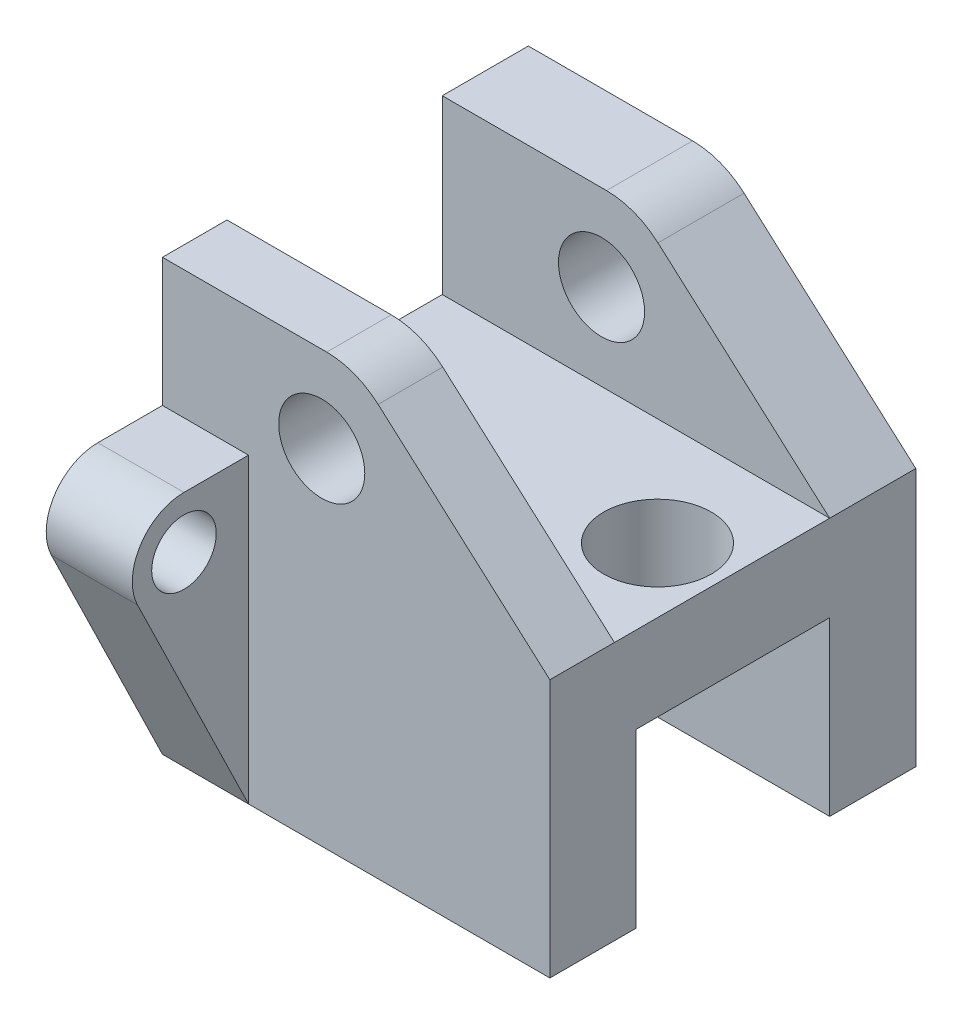
ISO-10303-21;
HEADER;
FILE_DESCRIPTION(('STEP AP214'),'2;1');
FILE_NAME('part.step','',(''),(''),'','','');
FILE_SCHEMA(('AUTOMOTIVE_DESIGN { 1 0 10303 214 1 1 1 1 }'));
ENDSEC;
DATA;
#1=APPLICATION_CONTEXT('core data for automotive mechanical design processes');
#2=APPLICATION_PROTOCOL_DEFINITION('international standard','automotive_design',2000,#1);
#3=PRODUCT_CONTEXT('',#1,'mechanical');
#4=PRODUCT('Part','Part','',(#3));
#5=PRODUCT_RELATED_PRODUCT_CATEGORY('part','',(#4));
#6=PRODUCT_DEFINITION_FORMATION('','',#4);
#7=PRODUCT_DEFINITION_CONTEXT('part definition',#1,'design');
#8=PRODUCT_DEFINITION('design','',#6,#7);
#9=PRODUCT_DEFINITION_SHAPE('','',#8);
#10=(LENGTH_UNIT() NAMED_UNIT(*) SI_UNIT(.MILLI.,.METRE.));
#11=(NAMED_UNIT(*) PLANE_ANGLE_UNIT() SI_UNIT($,.RADIAN.));
#12=(NAMED_UNIT(*) SI_UNIT($,.STERADIAN.) SOLID_ANGLE_UNIT());
#13=UNCERTAINTY_MEASURE_WITH_UNIT(LENGTH_MEASURE(1.E-05),#10,'distance_accuracy_value','');
#14=(GEOMETRIC_REPRESENTATION_CONTEXT(3) GLOBAL_UNCERTAINTY_ASSIGNED_CONTEXT((#13)) GLOBAL_UNIT_ASSIGNED_CONTEXT((#10,
#11,#12)) REPRESENTATION_CONTEXT('',''));
#15=CARTESIAN_POINT('',(0.,0.,0.));
#16=DIRECTION('',(0.,0.,1.));
#17=DIRECTION('',(1.,0.,0.));
#18=AXIS2_PLACEMENT_3D('',#15,#16,#17);
#19=CARTESIAN_POINT('',(0.,0.,42.5));
#20=DIRECTION('',(0.,0.,-1.));
#21=DIRECTION('',(-1.,0.,0.));
#22=AXIS2_PLACEMENT_3D('',#19,#20,#21);
#23=PLANE('',#22);
#24=CARTESIAN_POINT('',(-8.,20.,42.5));
#25=DIRECTION('',(0.,0.,1.));
#26=DIRECTION('',(1.,0.,0.));
#27=AXIS2_PLACEMENT_3D('',#24,#25,#26);
#28=CIRCLE('',#27,10.);
#29=CARTESIAN_POINT('',(2.00000000000001,20.,42.5));
#30=VERTEX_POINT('',#29);
#31=EDGE_CURVE('E244',#30,#30,#28,.T.);
#32=ORIENTED_EDGE('',*,*,#31,.F.);
#33=EDGE_LOOP('',(#32));
#34=FACE_BOUND('',#33,.T.);
#35=DIRECTION('',(-0.74740931868366,0.66436383882992,0.));
#36=VECTOR('',#35,1.);
#37=CARTESIAN_POINT('',(0.,40.,42.5));
#38=LINE('',#37,#36);
#39=CARTESIAN_POINT('',(45.,0.,42.5));
#40=VERTEX_POINT('',#39);
#41=CARTESIAN_POINT('',(5.11496129665589,35.4533677363059,42.5));
#42=VERTEX_POINT('',#41);
#43=EDGE_CURVE('E289',#40,#42,#38,.T.);
#44=ORIENTED_EDGE('',*,*,#43,.T.);
#45=CARTESIAN_POINT('',(-6.84358780228266,22.,42.5));
#46=DIRECTION('',(0.,0.,-1.));
#47=DIRECTION('',(-1.,0.,0.));
#48=AXIS2_PLACEMENT_3D('',#45,#46,#47);
#49=CIRCLE('',#48,18.);
#50=CARTESIAN_POINT('',(-6.84358780228266,40.,42.5));
#51=VERTEX_POINT('',#50);
#52=EDGE_CURVE('E11',#42,#51,#49,.F.);
#53=ORIENTED_EDGE('',*,*,#52,.T.);
#54=DIRECTION('',(-1.,0.,0.));
#55=VECTOR('',#54,1.);
#56=CARTESIAN_POINT('',(-45.,40.,42.5));
#57=LINE('',#56,#55);
#58=CARTESIAN_POINT('',(-45.,40.,42.5));
#59=VERTEX_POINT('',#58);
#60=EDGE_CURVE('E270',#51,#59,#57,.T.);
#61=ORIENTED_EDGE('',*,*,#60,.T.);
#62=DIRECTION('',(0.,-1.,0.));
#63=VECTOR('',#62,1.);
#64=CARTESIAN_POINT('',(-45.,0.,42.5));
#65=LINE('',#64,#63);
#66=CARTESIAN_POINT('',(-45.,10.1908003384835,42.5));
#67=VERTEX_POINT('',#66);
#68=EDGE_CURVE('E281',#59,#67,#65,.T.);
#69=ORIENTED_EDGE('',*,*,#68,.T.);
#70=DIRECTION('',(-1.,0.,0.));
#71=VECTOR('',#70,1.);
#72=CARTESIAN_POINT('',(-25.,10.1908003384835,42.5));
#73=LINE('',#72,#71);
#74=CARTESIAN_POINT('',(-25.,10.1908003384835,42.5));
#75=VERTEX_POINT('',#74);
#76=EDGE_CURVE('E348',#75,#67,#73,.T.);
#77=ORIENTED_EDGE('',*,*,#76,.F.);
#78=DIRECTION('',(0.,1.,0.));
#79=VECTOR('',#78,1.);
#80=CARTESIAN_POINT('',(-25.,0.,42.5));
#81=LINE('',#80,#79);
#82=CARTESIAN_POINT('',(-25.,-60.,42.5));
#83=VERTEX_POINT('',#82);
#84=EDGE_CURVE('E351',#83,#75,#81,.T.);
#85=ORIENTED_EDGE('',*,*,#84,.F.);
#86=DIRECTION('',(1.,0.,0.));
#87=VECTOR('',#86,1.);
#88=CARTESIAN_POINT('',(-45.,-60.,42.5));
#89=LINE('',#88,#87);
#90=CARTESIAN_POINT('',(45.,-60.,42.5));
#91=VERTEX_POINT('',#90);
#92=EDGE_CURVE('E282',#83,#91,#89,.T.);
#93=ORIENTED_EDGE('',*,*,#92,.T.);
#94=DIRECTION('',(0.,1.,0.));
#95=VECTOR('',#94,1.);
#96=CARTESIAN_POINT('',(45.,-60.,42.5));
#97=LINE('',#96,#95);
#98=EDGE_CURVE('E290',#91,#40,#97,.T.);
#99=ORIENTED_EDGE('',*,*,#98,.T.);
#100=EDGE_LOOP('',(#44,#53,#61,#69,#77,#85,#93,#99));
#101=FACE_BOUND('',#100,.T.);
#102=ADVANCED_FACE('F50',(#34,#101),#23,.F.);
#103=CARTESIAN_POINT('',(45.,-60.,22.5));
#104=DIRECTION('',(1.,0.,0.));
#105=DIRECTION('',(0.,0.,-1.));
#106=AXIS2_PLACEMENT_3D('',#103,#104,#105);
#107=PLANE('',#106);
#108=DIRECTION('',(0.,0.,-1.));
#109=VECTOR('',#108,1.);
#110=CARTESIAN_POINT('',(45.,-20.,0.));
#111=LINE('',#110,#109);
#112=CARTESIAN_POINT('',(45.,-20.,22.5));
#113=VERTEX_POINT('',#112);
#114=CARTESIAN_POINT('',(45.,-20.,-22.5));
#115=VERTEX_POINT('',#114);
#116=EDGE_CURVE('E350',#113,#115,#111,.T.);
#117=ORIENTED_EDGE('',*,*,#116,.T.);
#118=DIRECTION('',(0.,1.,0.));
#119=VECTOR('',#118,1.);
#120=CARTESIAN_POINT('',(45.,-60.,-22.5));
#121=LINE('',#120,#119);
#122=CARTESIAN_POINT('',(45.,-60.,-22.5));
#123=VERTEX_POINT('',#122);
#124=EDGE_CURVE('E207',#123,#115,#121,.T.);
#125=ORIENTED_EDGE('',*,*,#124,.F.);
#126=DIRECTION('',(0.,0.,-1.));
#127=VECTOR('',#126,1.);
#128=CARTESIAN_POINT('',(45.,-60.,22.5));
#129=LINE('',#128,#127);
#130=CARTESIAN_POINT('',(45.,-60.,-42.5));
#131=VERTEX_POINT('',#130);
#132=EDGE_CURVE('E212',#123,#131,#129,.T.);
#133=ORIENTED_EDGE('',*,*,#132,.T.);
#134=DIRECTION('',(0.,-1.,0.));
#135=VECTOR('',#134,1.);
#136=CARTESIAN_POINT('',(45.,0.,-42.5));
#137=LINE('',#136,#135);
#138=CARTESIAN_POINT('',(45.,0.,-42.5));
#139=VERTEX_POINT('',#138);
#140=EDGE_CURVE('E332',#139,#131,#137,.T.);
#141=ORIENTED_EDGE('',*,*,#140,.F.);
#142=DIRECTION('',(0.,0.,1.));
#143=VECTOR('',#142,1.);
#144=CARTESIAN_POINT('',(45.,0.,-42.5));
#145=LINE('',#144,#143);
#146=CARTESIAN_POINT('',(45.,0.,-22.5));
#147=VERTEX_POINT('',#146);
#148=EDGE_CURVE('E306',#139,#147,#145,.T.);
#149=ORIENTED_EDGE('',*,*,#148,.T.);
#150=DIRECTION('',(0.,0.,-1.));
#151=VECTOR('',#150,1.);
#152=CARTESIAN_POINT('',(45.,0.,22.5));
#153=LINE('',#152,#151);
#154=CARTESIAN_POINT('',(45.,0.,27.5));
#155=VERTEX_POINT('',#154);
#156=EDGE_CURVE('E231',#155,#147,#153,.T.);
#157=ORIENTED_EDGE('',*,*,#156,.F.);
#158=DIRECTION('',(0.,0.,-1.));
#159=VECTOR('',#158,1.);
#160=CARTESIAN_POINT('',(45.,0.,42.5));
#161=LINE('',#160,#159);
#162=EDGE_CURVE('E240',#40,#155,#161,.T.);
#163=ORIENTED_EDGE('',*,*,#162,.F.);
#164=ORIENTED_EDGE('',*,*,#98,.F.);
#165=CARTESIAN_POINT('',(45.,-60.,22.5));
#166=VERTEX_POINT('',#165);
#167=EDGE_CURVE('E230',#91,#166,#129,.T.);
#168=ORIENTED_EDGE('',*,*,#167,.T.);
#169=DIRECTION('',(0.,1.,0.));
#170=VECTOR('',#169,1.);
#171=CARTESIAN_POINT('',(45.,0.,22.5));
#172=LINE('',#171,#170);
#173=EDGE_CURVE('E345',#166,#113,#172,.T.);
#174=ORIENTED_EDGE('',*,*,#173,.T.);
#175=EDGE_LOOP('',(#117,#125,#133,#141,#149,#157,#163,#164,#168,#174));
#176=FACE_BOUND('',#175,.T.);
#177=ADVANCED_FACE('F297',(#176),#107,.T.);
#178=CARTESIAN_POINT('',(-45.,-60.,22.5));
#179=DIRECTION('',(-1.,0.,0.));
#180=DIRECTION('',(0.,0.,1.));
#181=AXIS2_PLACEMENT_3D('',#178,#179,#180);
#182=PLANE('',#181);
#183=DIRECTION('',(0.,1.,0.));
#184=VECTOR('',#183,1.);
#185=CARTESIAN_POINT('',(-45.,-60.,-22.5));
#186=LINE('',#185,#184);
#187=CARTESIAN_POINT('',(-45.,-60.,-22.5));
#188=VERTEX_POINT('',#187);
#189=CARTESIAN_POINT('',(-45.,-20.,-22.5));
#190=VERTEX_POINT('',#189);
#191=EDGE_CURVE('E192',#188,#190,#186,.T.);
#192=ORIENTED_EDGE('',*,*,#191,.T.);
#193=DIRECTION('',(0.,0.,-1.));
#194=VECTOR('',#193,1.);
#195=CARTESIAN_POINT('',(-45.,-20.,0.));
#196=LINE('',#195,#194);
#197=CARTESIAN_POINT('',(-45.,-20.,22.5));
#198=VERTEX_POINT('',#197);
#199=EDGE_CURVE('E346',#198,#190,#196,.T.);
#200=ORIENTED_EDGE('',*,*,#199,.F.);
#201=DIRECTION('',(0.,1.,0.));
#202=VECTOR('',#201,1.);
#203=CARTESIAN_POINT('',(-45.,0.,22.5));
#204=LINE('',#203,#202);
#205=CARTESIAN_POINT('',(-45.,-60.,22.5));
#206=VERTEX_POINT('',#205);
#207=EDGE_CURVE('E338',#206,#198,#204,.T.);
#208=ORIENTED_EDGE('',*,*,#207,.F.);
#209=DIRECTION('',(0.,0.,1.));
#210=VECTOR('',#209,1.);
#211=CARTESIAN_POINT('',(-45.,-60.,22.5));
#212=LINE('',#211,#210);
#213=CARTESIAN_POINT('',(-45.,-60.,42.5));
#214=VERTEX_POINT('',#213);
#215=EDGE_CURVE('E224',#206,#214,#212,.T.);
#216=ORIENTED_EDGE('',*,*,#215,.T.);
#217=DIRECTION('',(0.,-0.898996884493592,-0.437955022429033));
#218=VECTOR('',#217,1.);
#219=CARTESIAN_POINT('',(-45.,-28.2413846305098,57.9715164717117));
#220=LINE('',#219,#218);
#221=CARTESIAN_POINT('',(-45.,-7.06465993066494,68.2879626139231));
#222=VERTEX_POINT('',#221);
#223=EDGE_CURVE('E366',#222,#214,#220,.T.);
#224=ORIENTED_EDGE('',*,*,#223,.F.);
#225=CARTESIAN_POINT('',(-45.,-1.80919966151655,57.5));
#226=DIRECTION('',(-1.,0.,0.));
#227=DIRECTION('',(0.,0.,1.));
#228=AXIS2_PLACEMENT_3D('',#225,#226,#227);
#229=CIRCLE('',#228,12.);
#230=CARTESIAN_POINT('',(-45.,10.1908003384835,57.5));
#231=VERTEX_POINT('',#230);
#232=EDGE_CURVE('E361',#222,#231,#229,.T.);
#233=ORIENTED_EDGE('',*,*,#232,.T.);
#234=DIRECTION('',(0.,0.,-1.));
#235=VECTOR('',#234,1.);
#236=CARTESIAN_POINT('',(-45.,10.1908003384834,0.));
#237=LINE('',#236,#235);
#238=EDGE_CURVE('E360',#231,#67,#237,.T.);
#239=ORIENTED_EDGE('',*,*,#238,.T.);
#240=ORIENTED_EDGE('',*,*,#68,.F.);
#241=DIRECTION('',(0.,0.,-1.));
#242=VECTOR('',#241,1.);
#243=CARTESIAN_POINT('',(-45.,40.,42.5));
#244=LINE('',#243,#242);
#245=CARTESIAN_POINT('',(-45.,40.,27.5));
#246=VERTEX_POINT('',#245);
#247=EDGE_CURVE('E292',#59,#246,#244,.T.);
#248=ORIENTED_EDGE('',*,*,#247,.T.);
#249=DIRECTION('',(0.,1.,0.));
#250=VECTOR('',#249,1.);
#251=CARTESIAN_POINT('',(-45.,0.,27.5));
#252=LINE('',#251,#250);
#253=CARTESIAN_POINT('',(-45.,0.,27.5));
#254=VERTEX_POINT('',#253);
#255=EDGE_CURVE('E271',#254,#246,#252,.T.);
#256=ORIENTED_EDGE('',*,*,#255,.F.);
#257=DIRECTION('',(0.,0.,1.));
#258=VECTOR('',#257,1.);
#259=CARTESIAN_POINT('',(-45.,0.,22.5));
#260=LINE('',#259,#258);
#261=CARTESIAN_POINT('',(-45.,0.,-22.5));
#262=VERTEX_POINT('',#261);
#263=EDGE_CURVE('E239',#262,#254,#260,.T.);
#264=ORIENTED_EDGE('',*,*,#263,.F.);
#265=DIRECTION('',(0.,1.,0.));
#266=VECTOR('',#265,1.);
#267=CARTESIAN_POINT('',(-45.,0.,-22.5));
#268=LINE('',#267,#266);
#269=CARTESIAN_POINT('',(-45.,40.,-22.5));
#270=VERTEX_POINT('',#269);
#271=EDGE_CURVE('E324',#262,#270,#268,.T.);
#272=ORIENTED_EDGE('',*,*,#271,.T.);
#273=DIRECTION('',(0.,0.,1.));
#274=VECTOR('',#273,1.);
#275=CARTESIAN_POINT('',(-45.,40.,-42.5));
#276=LINE('',#275,#274);
#277=CARTESIAN_POINT('',(-45.,40.,-42.5));
#278=VERTEX_POINT('',#277);
#279=EDGE_CURVE('E312',#278,#270,#276,.T.);
#280=ORIENTED_EDGE('',*,*,#279,.F.);
#281=DIRECTION('',(0.,1.,0.));
#282=VECTOR('',#281,1.);
#283=CARTESIAN_POINT('',(-45.,-60.,-42.5));
#284=LINE('',#283,#282);
#285=CARTESIAN_POINT('',(-45.,12.,-42.5));
#286=VERTEX_POINT('',#285);
#287=EDGE_CURVE('E326',#286,#278,#284,.T.);
#288=ORIENTED_EDGE('',*,*,#287,.F.);
#289=DIRECTION('',(0.,0.,1.));
#290=VECTOR('',#289,1.);
#291=CARTESIAN_POINT('',(-45.,12.,0.));
#292=LINE('',#291,#290);
#293=CARTESIAN_POINT('',(-45.,12.,-57.5));
#294=VERTEX_POINT('',#293);
#295=EDGE_CURVE('E399',#294,#286,#292,.T.);
#296=ORIENTED_EDGE('',*,*,#295,.F.);
#297=CARTESIAN_POINT('',(-45.,0.,-57.5));
#298=DIRECTION('',(-1.,0.,0.));
#299=DIRECTION('',(0.,0.,1.));
#300=AXIS2_PLACEMENT_3D('',#297,#298,#299);
#301=CIRCLE('',#300,12.);
#302=CARTESIAN_POINT('',(-45.,-5.11394095286918,-68.3557638114767));
#303=VERTEX_POINT('',#302);
#304=EDGE_CURVE('E400',#294,#303,#301,.T.);
#305=ORIENTED_EDGE('',*,*,#304,.T.);
#306=DIRECTION('',(0.,-0.904646984289726,0.426161746072432));
#307=VECTOR('',#306,1.);
#308=CARTESIAN_POINT('',(-45.,-27.2816824111032,-57.9129683670853));
#309=LINE('',#308,#307);
#310=CARTESIAN_POINT('',(-45.,-60.,-42.5));
#311=VERTEX_POINT('',#310);
#312=EDGE_CURVE('E225',#303,#311,#309,.T.);
#313=ORIENTED_EDGE('',*,*,#312,.T.);
#314=EDGE_CURVE('E215',#311,#188,#212,.T.);
#315=ORIENTED_EDGE('',*,*,#314,.T.);
#316=EDGE_LOOP('',(#192,#200,#208,#216,#224,#233,#239,#240,#248,#256,#264,#272,#280,#288,#296,
#305,#313,#315));
#317=FACE_BOUND('',#316,.T.);
#318=CARTESIAN_POINT('',(-45.,-1.80919966151655,57.5));
#319=DIRECTION('',(-1.,0.,0.));
#320=DIRECTION('',(0.,0.,1.));
#321=AXIS2_PLACEMENT_3D('',#318,#319,#320);
#322=CIRCLE('',#321,7.50000000000001);
#323=CARTESIAN_POINT('',(-45.,-1.80919966151655,65.));
#324=VERTEX_POINT('',#323);
#325=EDGE_CURVE('E367',#324,#324,#322,.T.);
#326=ORIENTED_EDGE('',*,*,#325,.F.);
#327=EDGE_LOOP('',(#326));
#328=FACE_BOUND('',#327,.T.);
#329=CARTESIAN_POINT('',(-45.,0.,-57.5));
#330=DIRECTION('',(-1.,0.,0.));
#331=DIRECTION('',(0.,0.,1.));
#332=AXIS2_PLACEMENT_3D('',#329,#330,#331);
#333=CIRCLE('',#332,7.50000000000001);
#334=CARTESIAN_POINT('',(-45.,0.,-50.));
#335=VERTEX_POINT('',#334);
#336=EDGE_CURVE('E402',#335,#335,#333,.T.);
#337=ORIENTED_EDGE('',*,*,#336,.F.);
#338=EDGE_LOOP('',(#337));
#339=FACE_BOUND('',#338,.T.);
#340=ADVANCED_FACE('F217',(#317,#328,#339),#182,.T.);
#341=CARTESIAN_POINT('',(0.,-60.,0.));
#342=DIRECTION('',(0.,-1.,0.));
#343=DIRECTION('',(0.,0.,-1.));
#344=AXIS2_PLACEMENT_3D('',#341,#342,#343);
#345=PLANE('',#344);
#346=DIRECTION('',(1.,0.,0.));
#347=VECTOR('',#346,1.);
#348=CARTESIAN_POINT('',(-45.,-60.,-22.5));
#349=LINE('',#348,#347);
#350=EDGE_CURVE('E198',#188,#123,#349,.T.);
#351=ORIENTED_EDGE('',*,*,#350,.F.);
#352=ORIENTED_EDGE('',*,*,#314,.F.);
#353=DIRECTION('',(-1.,0.,0.));
#354=VECTOR('',#353,1.);
#355=CARTESIAN_POINT('',(-25.,-60.,-42.5));
#356=LINE('',#355,#354);
#357=CARTESIAN_POINT('',(-25.,-60.,-42.5));
#358=VERTEX_POINT('',#357);
#359=EDGE_CURVE('E391',#358,#311,#356,.T.);
#360=ORIENTED_EDGE('',*,*,#359,.F.);
#361=DIRECTION('',(-1.,0.,0.));
#362=VECTOR('',#361,1.);
#363=CARTESIAN_POINT('',(45.,-60.,-42.5));
#364=LINE('',#363,#362);
#365=EDGE_CURVE('E327',#131,#358,#364,.T.);
#366=ORIENTED_EDGE('',*,*,#365,.F.);
#367=ORIENTED_EDGE('',*,*,#132,.F.);
#368=EDGE_LOOP('',(#351,#352,#360,#366,#367));
#369=FACE_BOUND('',#368,.T.);
#370=ADVANCED_FACE('F214',(#369),#345,.T.);
#371=ORIENTED_EDGE('',*,*,#215,.F.);
#372=DIRECTION('',(1.,0.,0.));
#373=VECTOR('',#372,1.);
#374=CARTESIAN_POINT('',(-45.,-60.,22.5));
#375=LINE('',#374,#373);
#376=EDGE_CURVE('E340',#206,#166,#375,.T.);
#377=ORIENTED_EDGE('',*,*,#376,.T.);
#378=ORIENTED_EDGE('',*,*,#167,.F.);
#379=ORIENTED_EDGE('',*,*,#92,.F.);
#380=EDGE_CURVE('E283',#214,#83,#89,.T.);
#381=ORIENTED_EDGE('',*,*,#380,.F.);
#382=EDGE_LOOP('',(#371,#377,#378,#379,#381));
#383=FACE_BOUND('',#382,.T.);
#384=ADVANCED_FACE('F435',(#383),#345,.T.);
#385=CARTESIAN_POINT('',(0.,0.,0.));
#386=DIRECTION('',(0.,-1.,0.));
#387=DIRECTION('',(0.,0.,-1.));
#388=AXIS2_PLACEMENT_3D('',#385,#386,#387);
#389=PLANE('',#388);
#390=CARTESIAN_POINT('',(30.,0.,2.50000000000001));
#391=DIRECTION('',(0.,1.,0.));
#392=DIRECTION('',(0.,0.,1.));
#393=AXIS2_PLACEMENT_3D('',#390,#391,#392);
#394=CIRCLE('',#393,12.5);
#395=CARTESIAN_POINT('',(30.,0.,15.));
#396=VERTEX_POINT('',#395);
#397=EDGE_CURVE('E417',#396,#396,#394,.T.);
#398=ORIENTED_EDGE('',*,*,#397,.F.);
#399=EDGE_LOOP('',(#398));
#400=FACE_BOUND('',#399,.T.);
#401=ORIENTED_EDGE('',*,*,#156,.T.);
#402=DIRECTION('',(-1.,0.,0.));
#403=VECTOR('',#402,1.);
#404=CARTESIAN_POINT('',(-45.,0.,-22.5));
#405=LINE('',#404,#403);
#406=EDGE_CURVE('E236',#147,#262,#405,.T.);
#407=ORIENTED_EDGE('',*,*,#406,.T.);
#408=ORIENTED_EDGE('',*,*,#263,.T.);
#409=DIRECTION('',(-1.,0.,0.));
#410=VECTOR('',#409,1.);
#411=CARTESIAN_POINT('',(45.,0.,27.5));
#412=LINE('',#411,#410);
#413=EDGE_CURVE('E273',#155,#254,#412,.T.);
#414=ORIENTED_EDGE('',*,*,#413,.F.);
#415=EDGE_LOOP('',(#401,#407,#408,#414));
#416=FACE_BOUND('',#415,.T.);
#417=ADVANCED_FACE('F308',(#400,#416),#389,.F.);
#418=CARTESIAN_POINT('',(0.,40.,42.5));
#419=DIRECTION('',(-0.66436383882992,-0.74740931868366,0.));
#420=DIRECTION('',(0.74740931868366,-0.66436383882992,0.));
#421=AXIS2_PLACEMENT_3D('',#418,#419,#420);
#422=PLANE('',#421);
#423=DIRECTION('',(0.74740931868366,-0.66436383882992,0.));
#424=VECTOR('',#423,1.);
#425=CARTESIAN_POINT('',(0.,40.,27.5));
#426=LINE('',#425,#424);
#427=CARTESIAN_POINT('',(5.11496129665589,35.4533677363059,27.5));
#428=VERTEX_POINT('',#427);
#429=EDGE_CURVE('E298',#428,#155,#426,.T.);
#430=ORIENTED_EDGE('',*,*,#429,.F.);
#431=DIRECTION('',(0.,0.,-1.));
#432=VECTOR('',#431,1.);
#433=CARTESIAN_POINT('',(5.11496129665589,35.4533677363059,42.5));
#434=LINE('',#433,#432);
#435=EDGE_CURVE('E54',#428,#42,#434,.F.);
#436=ORIENTED_EDGE('',*,*,#435,.T.);
#437=ORIENTED_EDGE('',*,*,#43,.F.);
#438=ORIENTED_EDGE('',*,*,#162,.T.);
#439=EDGE_LOOP('',(#430,#436,#437,#438));
#440=FACE_BOUND('',#439,.T.);
#441=ADVANCED_FACE('F294',(#440),#422,.F.);
#442=CARTESIAN_POINT('',(-45.,40.,42.5));
#443=DIRECTION('',(0.,-1.,0.));
#444=DIRECTION('',(0.,0.,-1.));
#445=AXIS2_PLACEMENT_3D('',#442,#443,#444);
#446=PLANE('',#445);
#447=ORIENTED_EDGE('',*,*,#60,.F.);
#448=DIRECTION('',(0.,0.,-1.));
#449=VECTOR('',#448,1.);
#450=CARTESIAN_POINT('',(-6.84358780228266,40.,42.5));
#451=LINE('',#450,#449);
#452=CARTESIAN_POINT('',(-6.84358780228266,40.,27.5));
#453=VERTEX_POINT('',#452);
#454=EDGE_CURVE('E256',#51,#453,#451,.T.);
#455=ORIENTED_EDGE('',*,*,#454,.T.);
#456=DIRECTION('',(1.,0.,0.));
#457=VECTOR('',#456,1.);
#458=CARTESIAN_POINT('',(-45.,40.,27.5));
#459=LINE('',#458,#457);
#460=EDGE_CURVE('E246',#246,#453,#459,.T.);
#461=ORIENTED_EDGE('',*,*,#460,.F.);
#462=ORIENTED_EDGE('',*,*,#247,.F.);
#463=EDGE_LOOP('',(#447,#455,#461,#462));
#464=FACE_BOUND('',#463,.T.);
#465=ADVANCED_FACE('F263',(#464),#446,.F.);
#466=CARTESIAN_POINT('',(-8.,20.,42.5));
#467=DIRECTION('',(0.,0.,-1.));
#468=DIRECTION('',(-1.,0.,0.));
#469=AXIS2_PLACEMENT_3D('',#466,#467,#468);
#470=CYLINDRICAL_SURFACE('',#469,10.);
#471=CARTESIAN_POINT('',(-8.,20.,27.5));
#472=DIRECTION('',(0.,0.,1.));
#473=DIRECTION('',(1.,0.,0.));
#474=AXIS2_PLACEMENT_3D('',#471,#472,#473);
#475=CIRCLE('',#474,10.);
#476=CARTESIAN_POINT('',(2.00000000000001,20.,27.5));
#477=VERTEX_POINT('',#476);
#478=EDGE_CURVE('E245',#477,#477,#475,.T.);
#479=ORIENTED_EDGE('',*,*,#478,.F.);
#480=EDGE_LOOP('',(#479));
#481=FACE_BOUND('',#480,.T.);
#482=ORIENTED_EDGE('',*,*,#31,.T.);
#483=EDGE_LOOP('',(#482));
#484=FACE_BOUND('',#483,.T.);
#485=ADVANCED_FACE('F469',(#481,#484),#470,.F.);
#486=CARTESIAN_POINT('',(0.,0.,27.5));
#487=DIRECTION('',(0.,0.,1.));
#488=DIRECTION('',(1.,0.,0.));
#489=AXIS2_PLACEMENT_3D('',#486,#487,#488);
#490=PLANE('',#489);
#491=ORIENTED_EDGE('',*,*,#478,.T.);
#492=EDGE_LOOP('',(#491));
#493=FACE_BOUND('',#492,.T.);
#494=ORIENTED_EDGE('',*,*,#460,.T.);
#495=CARTESIAN_POINT('',(-6.84358780228266,22.,27.5));
#496=DIRECTION('',(0.,0.,1.));
#497=DIRECTION('',(1.,0.,0.));
#498=AXIS2_PLACEMENT_3D('',#495,#496,#497);
#499=CIRCLE('',#498,18.);
#500=EDGE_CURVE('E68',#453,#428,#499,.F.);
#501=ORIENTED_EDGE('',*,*,#500,.T.);
#502=ORIENTED_EDGE('',*,*,#429,.T.);
#503=ORIENTED_EDGE('',*,*,#413,.T.);
#504=ORIENTED_EDGE('',*,*,#255,.T.);
#505=EDGE_LOOP('',(#494,#501,#502,#503,#504));
#506=FACE_BOUND('',#505,.T.);
#507=ADVANCED_FACE('F266',(#493,#506),#490,.F.);
#508=CARTESIAN_POINT('',(0.,40.,-42.5));
#509=DIRECTION('',(-0.66436383882992,-0.74740931868366,0.));
#510=DIRECTION('',(0.74740931868366,-0.66436383882992,0.));
#511=AXIS2_PLACEMENT_3D('',#508,#509,#510);
#512=PLANE('',#511);
#513=DIRECTION('',(0.74740931868366,-0.66436383882992,0.));
#514=VECTOR('',#513,1.);
#515=CARTESIAN_POINT('',(0.,40.,-42.5));
#516=LINE('',#515,#514);
#517=CARTESIAN_POINT('',(5.11496129665588,35.4533677363059,-42.5));
#518=VERTEX_POINT('',#517);
#519=EDGE_CURVE('E318',#518,#139,#516,.T.);
#520=ORIENTED_EDGE('',*,*,#519,.F.);
#521=DIRECTION('',(0.,0.,1.));
#522=VECTOR('',#521,1.);
#523=CARTESIAN_POINT('',(5.11496129665588,35.4533677363059,-42.5));
#524=LINE('',#523,#522);
#525=CARTESIAN_POINT('',(5.11496129665588,35.4533677363059,-22.5));
#526=VERTEX_POINT('',#525);
#527=EDGE_CURVE('E223',#518,#526,#524,.T.);
#528=ORIENTED_EDGE('',*,*,#527,.T.);
#529=DIRECTION('',(0.74740931868366,-0.66436383882992,0.));
#530=VECTOR('',#529,1.);
#531=CARTESIAN_POINT('',(0.,40.,-22.5));
#532=LINE('',#531,#530);
#533=EDGE_CURVE('E248',#526,#147,#532,.T.);
#534=ORIENTED_EDGE('',*,*,#533,.T.);
#535=ORIENTED_EDGE('',*,*,#148,.F.);
#536=EDGE_LOOP('',(#520,#528,#534,#535));
#537=FACE_BOUND('',#536,.T.);
#538=ADVANCED_FACE('F707',(#537),#512,.F.);
#539=CARTESIAN_POINT('',(-45.,40.,-42.5));
#540=DIRECTION('',(0.,-1.,0.));
#541=DIRECTION('',(0.,0.,-1.));
#542=AXIS2_PLACEMENT_3D('',#539,#540,#541);
#543=PLANE('',#542);
#544=DIRECTION('',(1.,0.,0.));
#545=VECTOR('',#544,1.);
#546=CARTESIAN_POINT('',(-45.,40.,-22.5));
#547=LINE('',#546,#545);
#548=CARTESIAN_POINT('',(-6.84358780228269,40.,-22.5));
#549=VERTEX_POINT('',#548);
#550=EDGE_CURVE('E320',#270,#549,#547,.T.);
#551=ORIENTED_EDGE('',*,*,#550,.T.);
#552=DIRECTION('',(0.,0.,1.));
#553=VECTOR('',#552,1.);
#554=CARTESIAN_POINT('',(-6.84358780228268,40.,-42.5));
#555=LINE('',#554,#553);
#556=CARTESIAN_POINT('',(-6.84358780228269,40.,-42.5));
#557=VERTEX_POINT('',#556);
#558=EDGE_CURVE('E254',#549,#557,#555,.F.);
#559=ORIENTED_EDGE('',*,*,#558,.T.);
#560=DIRECTION('',(1.,0.,0.));
#561=VECTOR('',#560,1.);
#562=CARTESIAN_POINT('',(-45.,40.,-42.5));
#563=LINE('',#562,#561);
#564=EDGE_CURVE('E317',#278,#557,#563,.T.);
#565=ORIENTED_EDGE('',*,*,#564,.F.);
#566=ORIENTED_EDGE('',*,*,#279,.T.);
#567=EDGE_LOOP('',(#551,#559,#565,#566));
#568=FACE_BOUND('',#567,.T.);
#569=ADVANCED_FACE('F700',(#568),#543,.F.);
#570=CARTESIAN_POINT('',(0.,0.,-42.5));
#571=DIRECTION('',(0.,0.,-1.));
#572=DIRECTION('',(-1.,0.,0.));
#573=AXIS2_PLACEMENT_3D('',#570,#571,#572);
#574=PLANE('',#573);
#575=ORIENTED_EDGE('',*,*,#564,.T.);
#576=CARTESIAN_POINT('',(-6.84358780228267,22.,-42.5));
#577=DIRECTION('',(0.,0.,-1.));
#578=DIRECTION('',(-1.,0.,0.));
#579=AXIS2_PLACEMENT_3D('',#576,#577,#578);
#580=CIRCLE('',#579,18.);
#581=EDGE_CURVE('E253',#557,#518,#580,.T.);
#582=ORIENTED_EDGE('',*,*,#581,.T.);
#583=ORIENTED_EDGE('',*,*,#519,.T.);
#584=ORIENTED_EDGE('',*,*,#140,.T.);
#585=ORIENTED_EDGE('',*,*,#365,.T.);
#586=DIRECTION('',(0.,-1.,0.));
#587=VECTOR('',#586,1.);
#588=CARTESIAN_POINT('',(-25.,0.,-42.5));
#589=LINE('',#588,#587);
#590=CARTESIAN_POINT('',(-25.,12.,-42.5));
#591=VERTEX_POINT('',#590);
#592=EDGE_CURVE('E388',#591,#358,#589,.T.);
#593=ORIENTED_EDGE('',*,*,#592,.F.);
#594=DIRECTION('',(-1.,0.,0.));
#595=VECTOR('',#594,1.);
#596=CARTESIAN_POINT('',(-25.,12.,-42.5));
#597=LINE('',#596,#595);
#598=EDGE_CURVE('E375',#591,#286,#597,.T.);
#599=ORIENTED_EDGE('',*,*,#598,.T.);
#600=ORIENTED_EDGE('',*,*,#287,.T.);
#601=EDGE_LOOP('',(#575,#582,#583,#584,#585,#593,#599,#600));
#602=FACE_BOUND('',#601,.T.);
#603=CARTESIAN_POINT('',(-8.,20.,-42.5));
#604=DIRECTION('',(0.,0.,1.));
#605=DIRECTION('',(1.,0.,0.));
#606=AXIS2_PLACEMENT_3D('',#603,#604,#605);
#607=CIRCLE('',#606,10.);
#608=CARTESIAN_POINT('',(2.00000000000001,20.,-42.5));
#609=VERTEX_POINT('',#608);
#610=EDGE_CURVE('E249',#609,#609,#607,.T.);
#611=ORIENTED_EDGE('',*,*,#610,.T.);
#612=EDGE_LOOP('',(#611));
#613=FACE_BOUND('',#612,.T.);
#614=ADVANCED_FACE('F686',(#602,#613),#574,.T.);
#615=CARTESIAN_POINT('',(0.,0.,-22.5));
#616=DIRECTION('',(0.,0.,-1.));
#617=DIRECTION('',(-1.,0.,0.));
#618=AXIS2_PLACEMENT_3D('',#615,#616,#617);
#619=PLANE('',#618);
#620=CARTESIAN_POINT('',(-8.,20.,-22.5));
#621=DIRECTION('',(0.,0.,-1.));
#622=DIRECTION('',(-1.,0.,0.));
#623=AXIS2_PLACEMENT_3D('',#620,#621,#622);
#624=CIRCLE('',#623,10.);
#625=CARTESIAN_POINT('',(-18.,20.,-22.5));
#626=VERTEX_POINT('',#625);
#627=EDGE_CURVE('E250',#626,#626,#624,.T.);
#628=ORIENTED_EDGE('',*,*,#627,.T.);
#629=EDGE_LOOP('',(#628));
#630=FACE_BOUND('',#629,.T.);
#631=ORIENTED_EDGE('',*,*,#533,.F.);
#632=CARTESIAN_POINT('',(-6.84358780228267,22.,-22.5));
#633=DIRECTION('',(0.,0.,-1.));
#634=DIRECTION('',(-1.,0.,0.));
#635=AXIS2_PLACEMENT_3D('',#632,#633,#634);
#636=CIRCLE('',#635,18.);
#637=EDGE_CURVE('E227',#526,#549,#636,.F.);
#638=ORIENTED_EDGE('',*,*,#637,.T.);
#639=ORIENTED_EDGE('',*,*,#550,.F.);
#640=ORIENTED_EDGE('',*,*,#271,.F.);
#641=ORIENTED_EDGE('',*,*,#406,.F.);
#642=EDGE_LOOP('',(#631,#638,#639,#640,#641));
#643=FACE_BOUND('',#642,.T.);
#644=ADVANCED_FACE('F678',(#630,#643),#619,.F.);
#645=CARTESIAN_POINT('',(-8.,20.,-42.5));
#646=DIRECTION('',(0.,0.,1.));
#647=DIRECTION('',(1.,0.,0.));
#648=AXIS2_PLACEMENT_3D('',#645,#646,#647);
#649=CYLINDRICAL_SURFACE('',#648,10.);
#650=ORIENTED_EDGE('',*,*,#610,.F.);
#651=EDGE_LOOP('',(#650));
#652=FACE_BOUND('',#651,.T.);
#653=ORIENTED_EDGE('',*,*,#627,.F.);
#654=EDGE_LOOP('',(#653));
#655=FACE_BOUND('',#654,.T.);
#656=ADVANCED_FACE('F621',(#652,#655),#649,.F.);
#657=CARTESIAN_POINT('',(-45.,0.,22.5));
#658=DIRECTION('',(0.,0.,-1.));
#659=DIRECTION('',(-1.,0.,0.));
#660=AXIS2_PLACEMENT_3D('',#657,#658,#659);
#661=PLANE('',#660);
#662=ORIENTED_EDGE('',*,*,#173,.F.);
#663=ORIENTED_EDGE('',*,*,#376,.F.);
#664=ORIENTED_EDGE('',*,*,#207,.T.);
#665=DIRECTION('',(1.,0.,0.));
#666=VECTOR('',#665,1.);
#667=CARTESIAN_POINT('',(-45.,-20.,22.5));
#668=LINE('',#667,#666);
#669=EDGE_CURVE('E336',#198,#113,#668,.T.);
#670=ORIENTED_EDGE('',*,*,#669,.T.);
#671=EDGE_LOOP('',(#662,#663,#664,#670));
#672=FACE_BOUND('',#671,.T.);
#673=ADVANCED_FACE('F498',(#672),#661,.T.);
#674=CARTESIAN_POINT('',(-45.,-20.,0.));
#675=DIRECTION('',(0.,-1.,0.));
#676=DIRECTION('',(0.,0.,-1.));
#677=AXIS2_PLACEMENT_3D('',#674,#675,#676);
#678=PLANE('',#677);
#679=CARTESIAN_POINT('',(30.,-20.,2.50000000000001));
#680=DIRECTION('',(0.,1.,0.));
#681=DIRECTION('',(0.,0.,1.));
#682=AXIS2_PLACEMENT_3D('',#679,#680,#681);
#683=CIRCLE('',#682,12.5);
#684=CARTESIAN_POINT('',(30.,-20.,15.));
#685=VERTEX_POINT('',#684);
#686=EDGE_CURVE('E404',#685,#685,#683,.T.);
#687=ORIENTED_EDGE('',*,*,#686,.T.);
#688=EDGE_LOOP('',(#687));
#689=FACE_BOUND('',#688,.T.);
#690=ORIENTED_EDGE('',*,*,#116,.F.);
#691=ORIENTED_EDGE('',*,*,#669,.F.);
#692=ORIENTED_EDGE('',*,*,#199,.T.);
#693=DIRECTION('',(1.,0.,0.));
#694=VECTOR('',#693,1.);
#695=CARTESIAN_POINT('',(-45.,-20.,-22.5));
#696=LINE('',#695,#694);
#697=EDGE_CURVE('E205',#190,#115,#696,.T.);
#698=ORIENTED_EDGE('',*,*,#697,.T.);
#699=EDGE_LOOP('',(#690,#691,#692,#698));
#700=FACE_BOUND('',#699,.T.);
#701=ADVANCED_FACE('F424',(#689,#700),#678,.T.);
#702=CARTESIAN_POINT('',(-25.,-28.2413846305098,57.9715164717117));
#703=DIRECTION('',(0.,0.437955022429033,-0.898996884493592));
#704=DIRECTION('',(0.,0.898996884493592,0.437955022429033));
#705=AXIS2_PLACEMENT_3D('',#702,#703,#704);
#706=PLANE('',#705);
#707=ORIENTED_EDGE('',*,*,#223,.T.);
#708=ORIENTED_EDGE('',*,*,#380,.T.);
#709=DIRECTION('',(0.,-0.898996884493592,-0.437955022429033));
#710=VECTOR('',#709,1.);
#711=CARTESIAN_POINT('',(-25.,-28.2413846305098,57.9715164717117));
#712=LINE('',#711,#710);
#713=CARTESIAN_POINT('',(-25.,-7.06465993066494,68.2879626139231));
#714=VERTEX_POINT('',#713);
#715=EDGE_CURVE('E382',#714,#83,#712,.T.);
#716=ORIENTED_EDGE('',*,*,#715,.F.);
#717=DIRECTION('',(-1.,0.,0.));
#718=VECTOR('',#717,1.);
#719=CARTESIAN_POINT('',(-25.,-7.06465993066494,68.2879626139231));
#720=LINE('',#719,#718);
#721=EDGE_CURVE('E355',#714,#222,#720,.T.);
#722=ORIENTED_EDGE('',*,*,#721,.T.);
#723=EDGE_LOOP('',(#707,#708,#716,#722));
#724=FACE_BOUND('',#723,.T.);
#725=ADVANCED_FACE('F440',(#724),#706,.F.);
#726=CARTESIAN_POINT('',(-25.,10.1908003384834,0.));
#727=DIRECTION('',(0.,1.,0.));
#728=DIRECTION('',(0.,0.,1.));
#729=AXIS2_PLACEMENT_3D('',#726,#727,#728);
#730=PLANE('',#729);
#731=ORIENTED_EDGE('',*,*,#238,.F.);
#732=DIRECTION('',(-1.,0.,0.));
#733=VECTOR('',#732,1.);
#734=CARTESIAN_POINT('',(-25.,10.1908003384835,57.5));
#735=LINE('',#734,#733);
#736=CARTESIAN_POINT('',(-25.,10.1908003384835,57.5));
#737=VERTEX_POINT('',#736);
#738=EDGE_CURVE('E354',#737,#231,#735,.T.);
#739=ORIENTED_EDGE('',*,*,#738,.F.);
#740=DIRECTION('',(0.,0.,-1.));
#741=VECTOR('',#740,1.);
#742=CARTESIAN_POINT('',(-25.,10.1908003384834,0.));
#743=LINE('',#742,#741);
#744=EDGE_CURVE('E374',#737,#75,#743,.T.);
#745=ORIENTED_EDGE('',*,*,#744,.T.);
#746=ORIENTED_EDGE('',*,*,#76,.T.);
#747=EDGE_LOOP('',(#731,#739,#745,#746));
#748=FACE_BOUND('',#747,.T.);
#749=ADVANCED_FACE('F444',(#748),#730,.T.);
#750=CARTESIAN_POINT('',(-25.,-1.80919966151655,57.5));
#751=DIRECTION('',(-1.,0.,0.));
#752=DIRECTION('',(0.,0.,1.));
#753=AXIS2_PLACEMENT_3D('',#750,#751,#752);
#754=CYLINDRICAL_SURFACE('',#753,7.50000000000001);
#755=CARTESIAN_POINT('',(-25.,-1.80919966151655,57.5));
#756=DIRECTION('',(-1.,0.,0.));
#757=DIRECTION('',(0.,0.,1.));
#758=AXIS2_PLACEMENT_3D('',#755,#756,#757);
#759=CIRCLE('',#758,7.50000000000001);
#760=CARTESIAN_POINT('',(-25.,-1.80919966151655,65.));
#761=VERTEX_POINT('',#760);
#762=EDGE_CURVE('E365',#761,#761,#759,.T.);
#763=ORIENTED_EDGE('',*,*,#762,.F.);
#764=EDGE_LOOP('',(#763));
#765=FACE_BOUND('',#764,.T.);
#766=ORIENTED_EDGE('',*,*,#325,.T.);
#767=EDGE_LOOP('',(#766));
#768=FACE_BOUND('',#767,.T.);
#769=ADVANCED_FACE('F582',(#765,#768),#754,.F.);
#770=CARTESIAN_POINT('',(-25.,-1.80919966151655,57.5));
#771=DIRECTION('',(-1.,0.,0.));
#772=DIRECTION('',(0.,0.,1.));
#773=AXIS2_PLACEMENT_3D('',#770,#771,#772);
#774=CYLINDRICAL_SURFACE('',#773,12.);
#775=ORIENTED_EDGE('',*,*,#232,.F.);
#776=ORIENTED_EDGE('',*,*,#721,.F.);
#777=CARTESIAN_POINT('',(-25.,-1.80919966151655,57.5));
#778=DIRECTION('',(-1.,0.,0.));
#779=DIRECTION('',(0.,0.,1.));
#780=AXIS2_PLACEMENT_3D('',#777,#778,#779);
#781=CIRCLE('',#780,12.);
#782=EDGE_CURVE('E377',#714,#737,#781,.T.);
#783=ORIENTED_EDGE('',*,*,#782,.T.);
#784=ORIENTED_EDGE('',*,*,#738,.T.);
#785=EDGE_LOOP('',(#775,#776,#783,#784));
#786=FACE_BOUND('',#785,.T.);
#787=ADVANCED_FACE('F439',(#786),#774,.T.);
#788=CARTESIAN_POINT('',(-25.,0.,0.));
#789=DIRECTION('',(-1.,0.,0.));
#790=DIRECTION('',(0.,0.,1.));
#791=AXIS2_PLACEMENT_3D('',#788,#789,#790);
#792=PLANE('',#791);
#793=ORIENTED_EDGE('',*,*,#762,.T.);
#794=EDGE_LOOP('',(#793));
#795=FACE_BOUND('',#794,.T.);
#796=ORIENTED_EDGE('',*,*,#715,.T.);
#797=ORIENTED_EDGE('',*,*,#84,.T.);
#798=ORIENTED_EDGE('',*,*,#744,.F.);
#799=ORIENTED_EDGE('',*,*,#782,.F.);
#800=EDGE_LOOP('',(#796,#797,#798,#799));
#801=FACE_BOUND('',#800,.T.);
#802=ADVANCED_FACE('F567',(#795,#801),#792,.F.);
#803=CARTESIAN_POINT('',(-25.,12.,0.));
#804=DIRECTION('',(0.,-1.,0.));
#805=DIRECTION('',(0.,0.,-1.));
#806=AXIS2_PLACEMENT_3D('',#803,#804,#805);
#807=PLANE('',#806);
#808=ORIENTED_EDGE('',*,*,#295,.T.);
#809=ORIENTED_EDGE('',*,*,#598,.F.);
#810=DIRECTION('',(0.,0.,1.));
#811=VECTOR('',#810,1.);
#812=CARTESIAN_POINT('',(-25.,12.,0.));
#813=LINE('',#812,#811);
#814=CARTESIAN_POINT('',(-25.,12.,-57.5));
#815=VERTEX_POINT('',#814);
#816=EDGE_CURVE('E415',#815,#591,#813,.T.);
#817=ORIENTED_EDGE('',*,*,#816,.F.);
#818=DIRECTION('',(-1.,0.,0.));
#819=VECTOR('',#818,1.);
#820=CARTESIAN_POINT('',(-25.,12.,-57.5));
#821=LINE('',#820,#819);
#822=EDGE_CURVE('E389',#815,#294,#821,.T.);
#823=ORIENTED_EDGE('',*,*,#822,.T.);
#824=EDGE_LOOP('',(#808,#809,#817,#823));
#825=FACE_BOUND('',#824,.T.);
#826=ADVANCED_FACE('F561',(#825),#807,.F.);
#827=CARTESIAN_POINT('',(-25.,-27.2816824111032,-57.9129683670853));
#828=DIRECTION('',(0.,-0.426161746072432,-0.904646984289726));
#829=DIRECTION('',(0.,0.904646984289726,-0.426161746072432));
#830=AXIS2_PLACEMENT_3D('',#827,#828,#829);
#831=PLANE('',#830);
#832=ORIENTED_EDGE('',*,*,#312,.F.);
#833=DIRECTION('',(-1.,0.,0.));
#834=VECTOR('',#833,1.);
#835=CARTESIAN_POINT('',(-25.,-5.11394095286918,-68.3557638114767));
#836=LINE('',#835,#834);
#837=CARTESIAN_POINT('',(-25.,-5.11394095286918,-68.3557638114767));
#838=VERTEX_POINT('',#837);
#839=EDGE_CURVE('E390',#838,#303,#836,.T.);
#840=ORIENTED_EDGE('',*,*,#839,.F.);
#841=DIRECTION('',(0.,-0.904646984289726,0.426161746072432));
#842=VECTOR('',#841,1.);
#843=CARTESIAN_POINT('',(-25.,-27.2816824111032,-57.9129683670853));
#844=LINE('',#843,#842);
#845=EDGE_CURVE('E409',#838,#358,#844,.T.);
#846=ORIENTED_EDGE('',*,*,#845,.T.);
#847=ORIENTED_EDGE('',*,*,#359,.T.);
#848=EDGE_LOOP('',(#832,#840,#846,#847));
#849=FACE_BOUND('',#848,.T.);
#850=ADVANCED_FACE('F553',(#849),#831,.T.);
#851=CARTESIAN_POINT('',(-25.,0.,-57.5));
#852=DIRECTION('',(-1.,0.,0.));
#853=DIRECTION('',(0.,0.,1.));
#854=AXIS2_PLACEMENT_3D('',#851,#852,#853);
#855=CYLINDRICAL_SURFACE('',#854,7.50000000000001);
#856=CARTESIAN_POINT('',(-25.,0.,-57.5));
#857=DIRECTION('',(-1.,0.,0.));
#858=DIRECTION('',(0.,0.,1.));
#859=AXIS2_PLACEMENT_3D('',#856,#857,#858);
#860=CIRCLE('',#859,7.50000000000001);
#861=CARTESIAN_POINT('',(-25.,0.,-50.));
#862=VERTEX_POINT('',#861);
#863=EDGE_CURVE('E397',#862,#862,#860,.T.);
#864=ORIENTED_EDGE('',*,*,#863,.F.);
#865=EDGE_LOOP('',(#864));
#866=FACE_BOUND('',#865,.T.);
#867=ORIENTED_EDGE('',*,*,#336,.T.);
#868=EDGE_LOOP('',(#867));
#869=FACE_BOUND('',#868,.T.);
#870=ADVANCED_FACE('F545',(#866,#869),#855,.F.);
#871=CARTESIAN_POINT('',(-25.,0.,-57.5));
#872=DIRECTION('',(-1.,0.,0.));
#873=DIRECTION('',(0.,0.,1.));
#874=AXIS2_PLACEMENT_3D('',#871,#872,#873);
#875=CYLINDRICAL_SURFACE('',#874,12.);
#876=ORIENTED_EDGE('',*,*,#304,.F.);
#877=ORIENTED_EDGE('',*,*,#822,.F.);
#878=CARTESIAN_POINT('',(-25.,0.,-57.5));
#879=DIRECTION('',(-1.,0.,0.));
#880=DIRECTION('',(0.,0.,1.));
#881=AXIS2_PLACEMENT_3D('',#878,#879,#880);
#882=CIRCLE('',#881,12.);
#883=EDGE_CURVE('E408',#815,#838,#882,.T.);
#884=ORIENTED_EDGE('',*,*,#883,.T.);
#885=ORIENTED_EDGE('',*,*,#839,.T.);
#886=EDGE_LOOP('',(#876,#877,#884,#885));
#887=FACE_BOUND('',#886,.T.);
#888=ADVANCED_FACE('F531',(#887),#875,.T.);
#889=CARTESIAN_POINT('',(-25.,0.,0.));
#890=DIRECTION('',(-1.,0.,0.));
#891=DIRECTION('',(0.,0.,1.));
#892=AXIS2_PLACEMENT_3D('',#889,#890,#891);
#893=PLANE('',#892);
#894=ORIENTED_EDGE('',*,*,#863,.T.);
#895=EDGE_LOOP('',(#894));
#896=FACE_BOUND('',#895,.T.);
#897=ORIENTED_EDGE('',*,*,#816,.T.);
#898=ORIENTED_EDGE('',*,*,#592,.T.);
#899=ORIENTED_EDGE('',*,*,#845,.F.);
#900=ORIENTED_EDGE('',*,*,#883,.F.);
#901=EDGE_LOOP('',(#897,#898,#899,#900));
#902=FACE_BOUND('',#901,.T.);
#903=ADVANCED_FACE('F523',(#896,#902),#893,.F.);
#904=CARTESIAN_POINT('',(30.,-20.,2.50000000000001));
#905=DIRECTION('',(0.,1.,0.));
#906=DIRECTION('',(0.,0.,1.));
#907=AXIS2_PLACEMENT_3D('',#904,#905,#906);
#908=CYLINDRICAL_SURFACE('',#907,12.5);
#909=ORIENTED_EDGE('',*,*,#686,.F.);
#910=EDGE_LOOP('',(#909));
#911=FACE_BOUND('',#910,.T.);
#912=ORIENTED_EDGE('',*,*,#397,.T.);
#913=EDGE_LOOP('',(#912));
#914=FACE_BOUND('',#913,.T.);
#915=ADVANCED_FACE('F456',(#911,#914),#908,.F.);
#916=CARTESIAN_POINT('',(-6.84358780228267,22.,-42.5));
#917=DIRECTION('',(0.,0.,1.));
#918=DIRECTION('',(1.,0.,0.));
#919=AXIS2_PLACEMENT_3D('',#916,#917,#918);
#920=CYLINDRICAL_SURFACE('',#919,18.);
#921=ORIENTED_EDGE('',*,*,#581,.F.);
#922=ORIENTED_EDGE('',*,*,#558,.F.);
#923=ORIENTED_EDGE('',*,*,#637,.F.);
#924=ORIENTED_EDGE('',*,*,#527,.F.);
#925=EDGE_LOOP('',(#921,#922,#923,#924));
#926=FACE_BOUND('',#925,.T.);
#927=ADVANCED_FACE('F446',(#926),#920,.T.);
#928=CARTESIAN_POINT('',(-6.84358780228266,22.,42.5));
#929=DIRECTION('',(0.,0.,-1.));
#930=DIRECTION('',(-1.,0.,0.));
#931=AXIS2_PLACEMENT_3D('',#928,#929,#930);
#932=CYLINDRICAL_SURFACE('',#931,18.);
#933=ORIENTED_EDGE('',*,*,#52,.F.);
#934=ORIENTED_EDGE('',*,*,#435,.F.);
#935=ORIENTED_EDGE('',*,*,#500,.F.);
#936=ORIENTED_EDGE('',*,*,#454,.F.);
#937=EDGE_LOOP('',(#933,#934,#935,#936));
#938=FACE_BOUND('',#937,.T.);
#939=ADVANCED_FACE('F47',(#938),#932,.T.);
#940=CARTESIAN_POINT('',(-45.,-60.,-22.5));
#941=DIRECTION('',(0.,0.,-1.));
#942=DIRECTION('',(-1.,0.,0.));
#943=AXIS2_PLACEMENT_3D('',#940,#941,#942);
#944=PLANE('',#943);
#945=ORIENTED_EDGE('',*,*,#124,.T.);
#946=ORIENTED_EDGE('',*,*,#697,.F.);
#947=ORIENTED_EDGE('',*,*,#191,.F.);
#948=ORIENTED_EDGE('',*,*,#350,.T.);
#949=EDGE_LOOP('',(#945,#946,#947,#948));
#950=FACE_BOUND('',#949,.T.);
#951=ADVANCED_FACE('F197',(#950),#944,.F.);
#952=CLOSED_SHELL('',(#102,#177,#340,#370,#384,#417,#441,#465,#485,#507,#538,#569,#614,#644,
#656,#673,#701,#725,#749,#769,#787,#802,#826,#850,#870,#888,#903,#915,#927,#939,#951));
#953=MANIFOLD_SOLID_BREP('B2',#952);
#954=ADVANCED_BREP_SHAPE_REPRESENTATION('',(#18,#953),#14);
#955=SHAPE_DEFINITION_REPRESENTATION(#9,#954);
ENDSEC;
END-ISO-10303-21;
